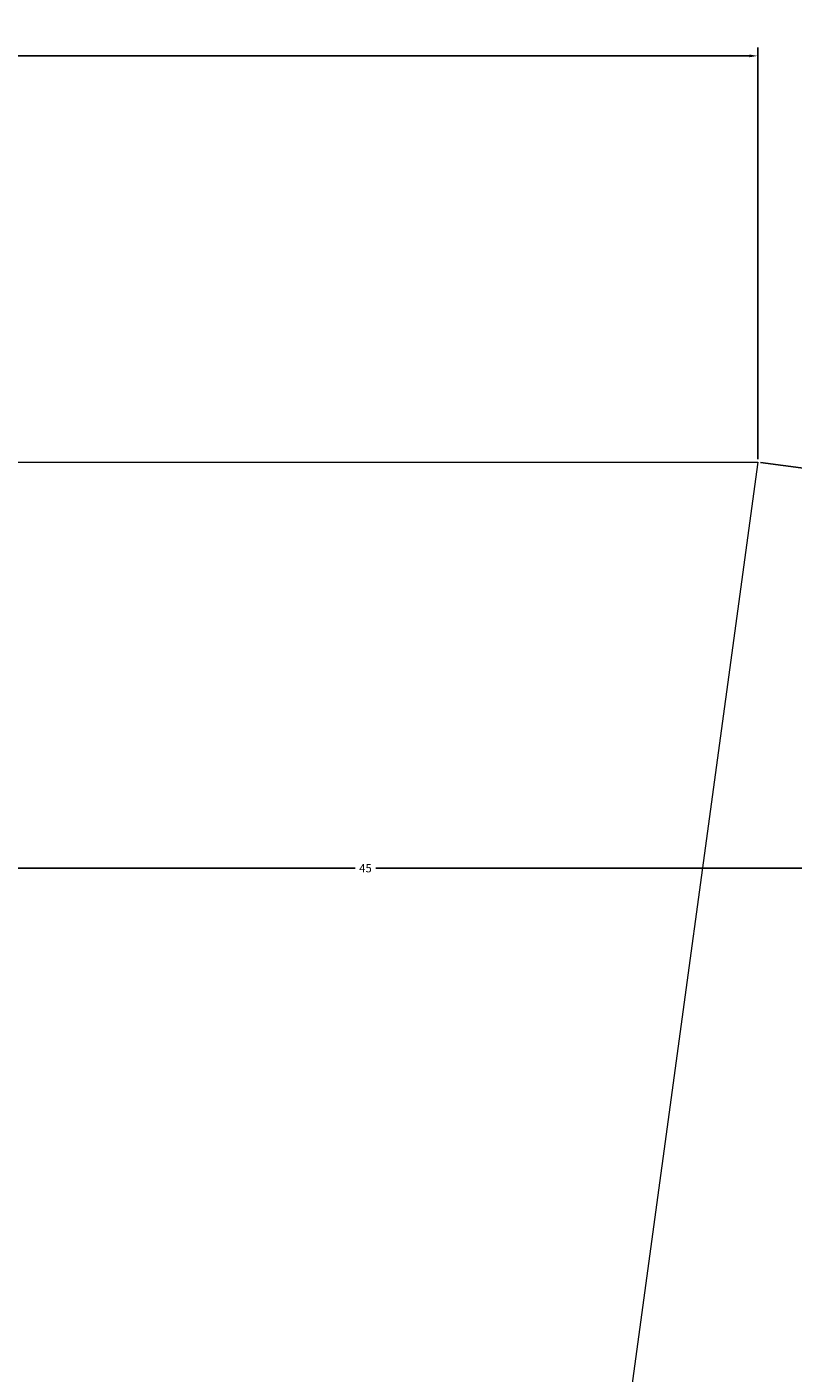
# Model space of a CAD drawing. Units: millimetres. Extents: x -9 to 135, y -119 to 27.
# Tile 8 of 12: x 78 to 95, y -18 to 11. Entities that reach past the tile are written whole.
import ezdxf

# ---------------------------------------------------------------- set-up
doc = ezdxf.new("R2010")
doc.units = ezdxf.units.MM
doc.layers.add('M-CONS', color=8, linetype='Continuous', lineweight=18)
doc.layers.add('M-DIMS', color=2, linetype='Continuous', lineweight=18)
doc.styles.get("Standard").update_dxf_attribs({"font": 'arial.ttf'})
doc.dimstyles.get("Standard").update_dxf_attribs({"dimtxt": 0.18, "dimasz": 0.18, "dimexe": 0.18, "dimexo": 0.0625, "dimgap": 0.09, "dimtad": 0, "dimtih": 1, "dimtoh": 1, "dimdec": 4, "dimzin": 0, "dimdsep": 46, "dimtxsty": 'Standard', "dimcen": 0.09, "dimadec": 0, "dimazin": 0, "dimtfac": 1, "dimtdec": 4, "dimtofl": 0, "dimtmove": 0, "dimatfit": 3, "dimfxl": 1, "dimtolj": 1, "dimtzin": 0, "dimarcsym": 0})

# ---------------------------------------------------------------- blocks, each defined once
blk = doc.blocks.new('*D2')
at = {"layer": 'Defpoints', "color": 0, "transparency": 16777216}
for p in [(126, 26.533), (0, 17.733), (126, 1.733)]:
    blk.add_point(p, dxfattribs=at)
at = {"layer": 'M-DIMS', "color": 0, "lineweight": -2, "transparency": 16777216}
for p, q in [((0, 17.796), (0, 26.713)), ((126, 1.796), (126, 26.713)), ((0.18, 26.533), (62.72, 26.533)), ((125.82, 26.533), (63.28, 26.533))]:
    blk.add_line(p, q, dxfattribs=at)
at = {"layer": 'M-DIMS', "color": 0, "transparency": 16777216}
for points in [[(0.18, 26.563), (0.18, 26.503), (0, 26.533)], [(125.82, 26.563), (125.82, 26.503), (126, 26.533)]]:
    blk.add_solid(points, dxfattribs=at)
at = {"layer": 'M-DIMS', "color": 0, "transparency": 16777216, "insert": (63, 26.533), "char_height": 0.18, "attachment_point": 5}
blk.add_mtext('\\A1;126', dxfattribs=at)
blk = doc.blocks.new('*D6')
at = {"layer": 'Defpoints', "color": 0, "transparency": 16777216}
for p in [(94, 10.533), (32, 1.733), (94, 1.733)]:
    blk.add_point(p, dxfattribs=at)
at = {"layer": 'M-DIMS', "color": 0, "lineweight": -2, "transparency": 16777216}
for p, q in [((32, 1.796), (32, 10.713)), ((32.18, 10.533), (62.782, 10.533)), ((93.82, 10.533), (63.218, 10.533)), ((94, 1.796), (94, 10.713))]:
    blk.add_line(p, q, dxfattribs=at)
at = {"layer": 'M-DIMS', "color": 0, "transparency": 16777216}
for points in [[(32.18, 10.563), (32.18, 10.503), (32, 10.533)], [(93.82, 10.563), (93.82, 10.503), (94, 10.533)]]:
    blk.add_solid(points, dxfattribs=at)
at = {"layer": 'M-DIMS', "color": 0, "transparency": 16777216, "insert": (63, 10.533), "char_height": 0.18, "attachment_point": 5}
blk.add_mtext('\\A1;62', dxfattribs=at)
blk = doc.blocks.new('*D10')
at = {"layer": 'Defpoints', "color": 0, "transparency": 16777216}
for p in [(63, 1.733), (108, 1.733), (63, -7.067)]:
    blk.add_point(p, dxfattribs=at)
at = {"layer": 'M-DIMS', "color": 0, "lineweight": -2, "transparency": 16777216}
for p, q in [((63, 1.671), (63, -7.247)), ((108, 1.671), (108, -7.247)), ((63.18, -7.067), (85.277, -7.067)), ((107.82, -7.067), (85.723, -7.067))]:
    blk.add_line(p, q, dxfattribs=at)
at = {"layer": 'M-DIMS', "color": 0, "transparency": 16777216}
for points in [[(63.18, -7.037), (63.18, -7.097), (63, -7.067)], [(107.82, -7.037), (107.82, -7.097), (108, -7.067)]]:
    blk.add_solid(points, dxfattribs=at)
at = {"layer": 'M-DIMS', "color": 0, "transparency": 16777216, "insert": (85.5, -7.067), "char_height": 0.18, "attachment_point": 5}
blk.add_mtext('\\A1;45', dxfattribs=at)
blk = doc.blocks.new('*D13')
at = {"layer": 'Defpoints', "color": 0, "transparency": 16777216}
for p in [(126, 1.733), (63, -92.267), (134.8, -92.267)]:
    blk.add_point(p, dxfattribs=at)
at = {"layer": 'M-DIMS', "color": 0, "lineweight": -2, "transparency": 16777216}
for p, q in [((126.062, 1.733), (134.98, 1.733)), ((134.8, 1.553), (134.8, -45.085)), ((134.8, -92.087), (134.8, -45.449)), ((63.063, -92.267), (134.98, -92.267))]:
    blk.add_line(p, q, dxfattribs=at)
at = {"layer": 'M-DIMS', "color": 0, "transparency": 16777216}
for points in [[(134.77, 1.553), (134.83, 1.553), (134.8, 1.733)], [(134.77, -92.087), (134.83, -92.087), (134.8, -92.267)]]:
    blk.add_solid(points, dxfattribs=at)
at = {"layer": 'M-DIMS', "color": 0, "transparency": 16777216, "insert": (134.8, -45.267), "char_height": 0.18, "attachment_point": 5}
blk.add_mtext('\\A1;94', dxfattribs=at)
blk = doc.blocks.new('*D15')
at = {"layer": 'Defpoints', "color": 0, "transparency": 16777216}
for p in [(94, 1.733), (80.835, -94.702), (89.554, -95.892)]:
    blk.add_point(p, dxfattribs=at)
at = {"layer": 'M-DIMS', "color": 0, "lineweight": -2, "transparency": 16777216}
for p, q in [((94.062, 1.725), (102.897, 0.519)), ((102.695, 0.365), (96.161, -47.493)), ((89.578, -95.714), (96.112, -47.856)), ((80.896, -94.71), (89.732, -95.916))]:
    blk.add_line(p, q, dxfattribs=at)
at = {"layer": 'M-DIMS', "color": 0, "transparency": 16777216}
for points in [[(102.665, 0.369), (102.724, 0.36), (102.719, 0.543)], [(89.548, -95.71), (89.608, -95.718), (89.554, -95.892)]]:
    blk.add_solid(points, dxfattribs=at)
at = {"layer": 'M-DIMS', "color": 0, "transparency": 16777216, "insert": (96.136, -47.675), "char_height": 0.18, "attachment_point": 5}
blk.add_mtext('\\A1;97.33', dxfattribs=at)
blk = doc.blocks.new('*D16')
at = {"layer": 'Defpoints', "color": 0, "transparency": 16777216}
for p in [(126, 1.733), (63, -92.267), (126, -119.067)]:
    blk.add_point(p, dxfattribs=at)
at = {"layer": 'M-DIMS', "color": 0, "lineweight": -2, "transparency": 16777216}
for p, q in [((126, 1.671), (126, -119.247)), ((63, -92.329), (63, -119.247)), ((63.18, -119.067), (94.281, -119.067)), ((125.82, -119.067), (94.719, -119.067))]:
    blk.add_line(p, q, dxfattribs=at)
at = {"layer": 'M-DIMS', "color": 0, "transparency": 16777216}
for points in [[(63.18, -119.037), (63.18, -119.097), (63, -119.067)], [(125.82, -119.037), (125.82, -119.097), (126, -119.067)]]:
    blk.add_solid(points, dxfattribs=at)
at = {"layer": 'M-DIMS', "color": 0, "transparency": 16777216, "insert": (94.5, -119.067), "char_height": 0.18, "attachment_point": 5}
blk.add_mtext('\\A1;63', dxfattribs=at)

msp = doc.modelspace()

# ---------------------------------------------------------------- linework, layer by layer
at = {"layer": 'M-CONS'}
for p, q in [((63, 1.733, 115.129), (94, 1.733, 115.129)), ((94, 1.733, 115.129), (80.835, -94.702, 115.129))]:
    msp.add_line(p, q, dxfattribs=at)

# ---------------------------------------------------------------- dimensions: what is measured, and where the dimension line sits
at = {"layer": 'M-DIMS'}
for base, p1, p2, picture, middle in [((126, 26.533), (0, 17.733), (126, 1.733), '*D2', (63, 26.533)), ((94, 10.533), (32, 1.733), (94, 1.733), '*D6', (63, 10.533)), ((126, -119.067), (63, -92.267), (126, 1.733), '*D16', (94.5, -119.067))]:
    dim = msp.add_linear_dim(base=base, p1=p1, p2=p2, dimstyle='Standard', override={"dimdec": 0, "dimlfac": 1, "dimrnd": 0, "dimzin": 0, "dimdsep": 46, "dimlunit": 2}, dxfattribs=at)
    dim.commit()
    dim.dimension.update_dxf_attribs({"geometry": picture, "text_midpoint": middle})
for base, p1, p2, angle, override, picture, middle in [((63, -7.067), (108, 1.733), (63, 1.733), 180, {"dimdec": 0, "dimlfac": 1, "dimrnd": 0, "dimzin": 0, "dimdsep": 46, "dimlunit": 2}, '*D10', (85.5, -7.067)), ((134.8, -92.267), (126, 1.733), (63, -92.267), 90, {"dimdec": 0, "dimlfac": 1, "dimrnd": 0, "dimzin": 0, "dimdsep": 46, "dimlunit": 2}, '*D13', (134.8, -45.267)), ((89.554, -95.892), (94, 1.733), (80.835, -94.702), 262.2259, {"dimdec": 2, "dimlfac": 1, "dimrnd": 0, "dimzin": 0, "dimdsep": 46, "dimlunit": 2}, '*D15', (96.136, -47.675))]:
    dim = msp.add_linear_dim(base=base, p1=p1, p2=p2, angle=angle, dimstyle='Standard', override=override, dxfattribs=at)
    dim.commit()
    dim.dimension.update_dxf_attribs({"geometry": picture, "text_midpoint": middle})

doc.saveas('drawing.dxf')
